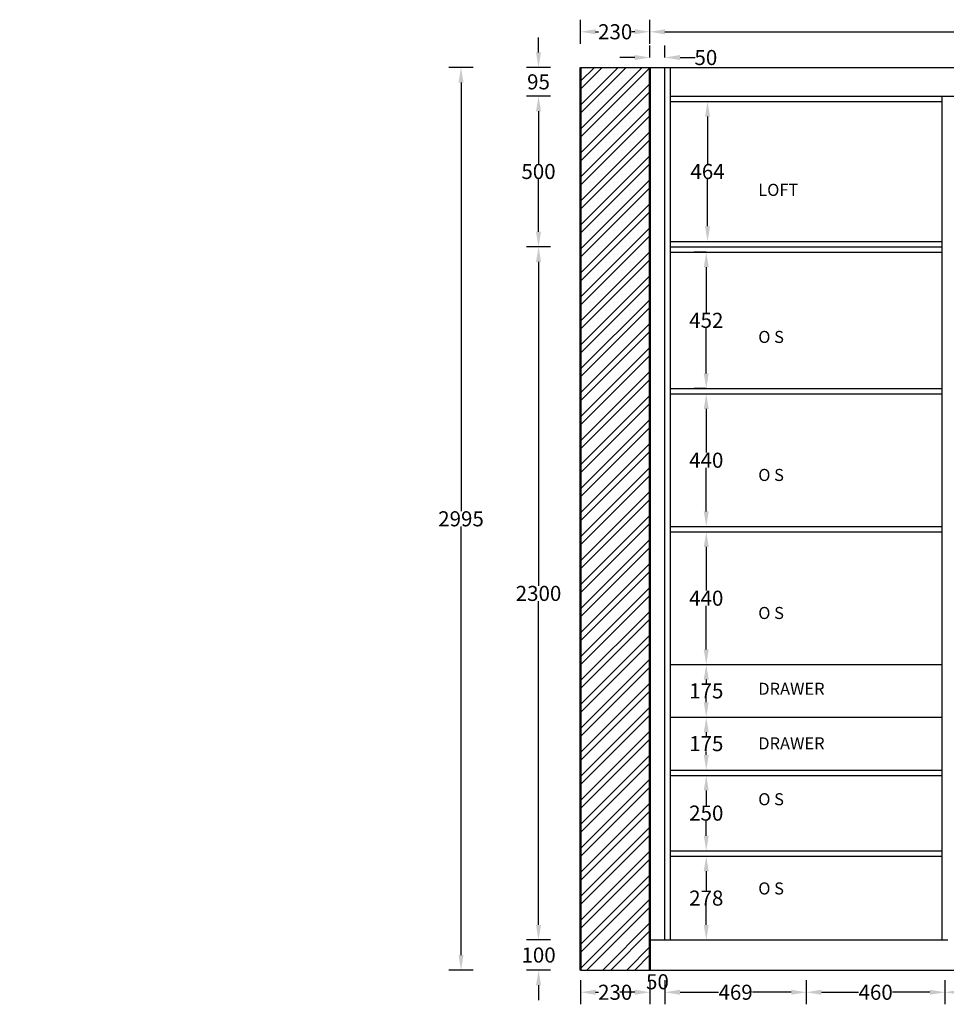
# Model space of a CAD drawing. Units: millimetres. Extents: x -472 to 16192, y -4730 to 4331.
# Tile 4 of 8: x 7860 to 10934, y -4399 to -1132. Entities that reach past the tile are written whole.
import ezdxf

# ---------------------------------------------------------------- set-up
doc = ezdxf.new("R2010")
doc.units = ezdxf.units.MM
doc.header["$MEASUREMENT"] = 0
for name, color, linetype, lineweight in [('A-ANNO-DIMS', 2, 'Continuous', 18), ('A-ANNO-TEXT', 6, 'Continuous', 18), ('A-ELEV', 7, 'Continuous', 25), ('A-WALL', 7, 'Continuous', 50), ('A-WALL-PATT', 8, 'Continuous', 13)]:
    doc.layers.add(name, color=color, linetype=linetype, lineweight=lineweight)
doc.styles.get("Standard").update_dxf_attribs({"font": 'arial.ttf'})
doc.dimstyles.get("Standard").update_dxf_attribs({"dimtxt": 50, "dimasz": 50, "dimexe": 40, "dimexo": 40, "dimgap": 0.09, "dimtad": 0, "dimtih": 1, "dimtoh": 1, "dimdec": 0, "dimzin": 0, "dimdsep": 46, "dimtxsty": 'Standard', "dimcen": 0.09, "dimclrd": 1, "dimclre": 3, "dimclrt": 6, "dimadec": 0, "dimazin": 0, "dimtfac": 1, "dimtdec": 0, "dimtofl": 0, "dimtmove": 0, "dimatfit": 3, "dimfxl": 40, "dimfxlon": 1, "dimtolj": 1, "dimtzin": 0, "dimarcsym": 0})

# ---------------------------------------------------------------- blocks, each defined once
blk = doc.blocks.new('*D44')
at = {"layer": 'A-ANNO-DIMS', "color": 0, "lineweight": -2, "transparency": 16777216}
for p, q in [((9950.7, -1212.4), (9950.7, -1132.4)), ((15090.7, -1212.4), (15090.7, -1132.4)), ((10000.7, -1172.4), (12446, -1172.4)), ((15040.7, -1172.4), (12595.3, -1172.4))]:
    blk.add_line(p, q, dxfattribs=at)
at = {"layer": 'A-ANNO-DIMS', "color": 0, "transparency": 16777216}
for points in [[(10000.7, -1164.1), (10000.7, -1180.8), (9950.7, -1172.4)], [(15040.7, -1164.1), (15040.7, -1180.8), (15090.7, -1172.4)]]:
    blk.add_solid(points, dxfattribs=at)
at = {"layer": 'Defpoints', "color": 0, "transparency": 16777216}
for p in [(15090.7, -1172.4), (9950.7, -1290.9), (15090.7, -1290.9)]:
    blk.add_point(p, dxfattribs=at)
at = {"layer": 'A-ANNO-DIMS', "color": 0, "transparency": 16777216, "insert": (12520.7, -1172.4), "char_height": 50, "attachment_point": 5}
blk.add_mtext('\\A1;5140', dxfattribs=at)
blk = doc.blocks.new('*D46')
at = {"layer": 'A-ANNO-DIMS', "color": 0, "lineweight": -2, "transparency": 16777216}
for p, q in [((9950.7, -1257.8), (9950.7, -1217.8)), ((10000.7, -1257.8), (10000.7, -1217.8)), ((9900.7, -1257.8), (9850.7, -1257.8)), ((10050.7, -1257.8), (10100.7, -1257.8))]:
    blk.add_line(p, q, dxfattribs=at)
at = {"layer": 'A-ANNO-DIMS', "color": 0, "transparency": 16777216}
for points in [[(9900.7, -1249.5), (9900.7, -1266.2), (9950.7, -1257.8)], [(10050.7, -1249.5), (10050.7, -1266.2), (10000.7, -1257.8)]]:
    blk.add_solid(points, dxfattribs=at)
at = {"layer": 'Defpoints', "color": 0, "transparency": 16777216}
for p in [(10000.7, -1257.8), (9950.7, -1290.9), (10000.7, -1290.9)]:
    blk.add_point(p, dxfattribs=at)
at = {"layer": 'A-ANNO-DIMS', "color": 0, "transparency": 16777216, "insert": (10136.5, -1257.8), "char_height": 50, "attachment_point": 5}
blk.add_mtext('\\A1;50', dxfattribs=at)
blk = doc.blocks.new('*D47')
at = {"layer": 'A-ANNO-DIMS', "color": 0, "lineweight": -2, "transparency": 16777216}
for p, q in [((9720.7, -1212.3), (9720.7, -1132.3)), ((9950.7, -1212.3), (9950.7, -1132.3)), ((9770.7, -1172.3), (9780, -1172.3)), ((9900.7, -1172.3), (9891.3, -1172.3))]:
    blk.add_line(p, q, dxfattribs=at)
at = {"layer": 'A-ANNO-DIMS', "color": 0, "transparency": 16777216}
for points in [[(9770.7, -1163.9), (9770.7, -1180.6), (9720.7, -1172.3)], [(9900.7, -1163.9), (9900.7, -1180.6), (9950.7, -1172.3)]]:
    blk.add_solid(points, dxfattribs=at)
at = {"layer": 'Defpoints', "color": 0, "transparency": 16777216}
for p in [(9950.7, -1172.3), (9720.7, -1290.9), (9950.7, -1290.9)]:
    blk.add_point(p, dxfattribs=at)
at = {"layer": 'A-ANNO-DIMS', "color": 0, "transparency": 16777216, "insert": (9835.7, -1172.3), "char_height": 50, "attachment_point": 5}
blk.add_mtext('\\A1;230', dxfattribs=at)
blk = doc.blocks.new('*D48')
at = {"layer": 'A-ANNO-DIMS', "color": 0, "lineweight": -2, "transparency": 16777216}
for p, q in [((9364.2, -1290.9), (9284.2, -1290.9)), ((9324.2, -1340.9), (9324.2, -2762.8)), ((9324.2, -4235.9), (9324.2, -2814)), ((9364.2, -4285.9), (9284.2, -4285.9))]:
    blk.add_line(p, q, dxfattribs=at)
at = {"layer": 'A-ANNO-DIMS', "color": 0, "transparency": 16777216}
for points in [[(9315.8, -1340.9), (9332.5, -1340.9), (9324.2, -1290.9)], [(9315.8, -4235.9), (9332.5, -4235.9), (9324.2, -4285.9)]]:
    blk.add_solid(points, dxfattribs=at)
at = {"layer": 'Defpoints', "color": 0, "transparency": 16777216}
for p in [(9720.7, -1290.9), (9324.2, -4285.9), (9720.7, -4285.9)]:
    blk.add_point(p, dxfattribs=at)
at = {"layer": 'A-ANNO-DIMS', "color": 0, "transparency": 16777216, "insert": (9324.2, -2788.4), "char_height": 50, "attachment_point": 5}
blk.add_mtext('\\A1;2995', dxfattribs=at)
blk = doc.blocks.new('*D49')
at = {"layer": 'A-ANNO-DIMS', "color": 0, "lineweight": -2, "transparency": 16777216}
for p, q in [((9581.5, -4135.9), (9581.5, -4085.9)), ((9621.5, -4185.9), (9541.5, -4185.9)), ((9621.5, -4285.9), (9541.5, -4285.9)), ((9581.5, -4335.9), (9581.5, -4385.9))]:
    blk.add_line(p, q, dxfattribs=at)
at = {"layer": 'A-ANNO-DIMS', "color": 0, "transparency": 16777216}
for points in [[(9573.1, -4135.9), (9589.8, -4135.9), (9581.5, -4185.9)], [(9573.1, -4335.9), (9589.8, -4335.9), (9581.5, -4285.9)]]:
    blk.add_solid(points, dxfattribs=at)
at = {"layer": 'Defpoints', "color": 0, "transparency": 16777216}
for p in [(9950.7, -4185.9), (9581.5, -4285.9), (9950.7, -4285.9)]:
    blk.add_point(p, dxfattribs=at)
at = {"layer": 'A-ANNO-DIMS', "color": 0, "transparency": 16777216, "insert": (9581.5, -4235.9), "char_height": 50, "attachment_point": 5}
blk.add_mtext('\\A1;100', dxfattribs=at)
blk = doc.blocks.new('*D50')
at = {"layer": 'A-ANNO-DIMS', "color": 0, "lineweight": -2, "transparency": 16777216}
for p, q in [((9621.3, -1885.9), (9541.3, -1885.9)), ((9581.3, -1935.9), (9581.3, -3010.3)), ((9581.3, -4135.9), (9581.3, -3061.5)), ((9621.3, -4185.9), (9541.3, -4185.9))]:
    blk.add_line(p, q, dxfattribs=at)
at = {"layer": 'A-ANNO-DIMS', "color": 0, "transparency": 16777216}
for points in [[(9573, -1935.9), (9589.6, -1935.9), (9581.3, -1885.9)], [(9573, -4135.9), (9589.6, -4135.9), (9581.3, -4185.9)]]:
    blk.add_solid(points, dxfattribs=at)
at = {"layer": 'Defpoints', "color": 0, "transparency": 16777216}
for p in [(9950.7, -1885.9), (9581.3, -4185.9), (9950.7, -4185.9)]:
    blk.add_point(p, dxfattribs=at)
at = {"layer": 'A-ANNO-DIMS', "color": 0, "transparency": 16777216, "insert": (9581.3, -3035.9), "char_height": 50, "attachment_point": 5}
blk.add_mtext('\\A1;2300', dxfattribs=at)
blk = doc.blocks.new('*D51')
at = {"layer": 'A-ANNO-DIMS', "color": 0, "lineweight": -2, "transparency": 16777216}
for p, q in [((9621.3, -1385.9), (9541.3, -1385.9)), ((9581.3, -1435.9), (9581.3, -1610.3)), ((9581.3, -1835.9), (9581.3, -1661.5)), ((9621.3, -1885.9), (9541.3, -1885.9))]:
    blk.add_line(p, q, dxfattribs=at)
at = {"layer": 'A-ANNO-DIMS', "color": 0, "transparency": 16777216}
for points in [[(9573, -1435.9), (9589.6, -1435.9), (9581.3, -1385.9)], [(9573, -1835.9), (9589.6, -1835.9), (9581.3, -1885.9)]]:
    blk.add_solid(points, dxfattribs=at)
at = {"layer": 'Defpoints', "color": 0, "transparency": 16777216}
for p in [(10018.7, -1385.9), (9581.3, -1885.9), (9950.7, -1885.9)]:
    blk.add_point(p, dxfattribs=at)
at = {"layer": 'A-ANNO-DIMS', "color": 0, "transparency": 16777216, "insert": (9581.3, -1635.9), "char_height": 50, "attachment_point": 5}
blk.add_mtext('\\A1;500', dxfattribs=at)
blk = doc.blocks.new('*D41')
at = {"layer": 'A-ANNO-DIMS', "color": 0, "lineweight": -2, "transparency": 16777216}
for p, q in [((9581.3, -1240.9), (9581.3, -1190.9)), ((9621.3, -1290.9), (9541.3, -1290.9)), ((9621.3, -1385.9), (9541.3, -1385.9)), ((9581.3, -1435.9), (9581.3, -1485.9))]:
    blk.add_line(p, q, dxfattribs=at)
at = {"layer": 'A-ANNO-DIMS', "color": 0, "transparency": 16777216}
for points in [[(9573, -1240.9), (9589.6, -1240.9), (9581.3, -1290.9)], [(9573, -1435.9), (9589.6, -1435.9), (9581.3, -1385.9)]]:
    blk.add_solid(points, dxfattribs=at)
at = {"layer": 'Defpoints', "color": 0, "transparency": 16777216}
for p in [(9950.7, -1290.9), (9581.3, -1385.9), (9950.7, -1385.9)]:
    blk.add_point(p, dxfattribs=at)
at = {"layer": 'A-ANNO-DIMS', "color": 0, "transparency": 16777216, "insert": (9581.3, -1338.4), "char_height": 50, "attachment_point": 5}
blk.add_mtext('\\A1;95', dxfattribs=at)
blk = doc.blocks.new('*D42')
at = {"layer": 'A-ANNO-DIMS', "color": 0, "lineweight": -2, "transparency": 16777216}
for p, q in [((9720.7, -4319.4), (9720.7, -4399.4)), ((9950.7, -4319.4), (9950.7, -4399.4)), ((9770.7, -4359.4), (9780, -4359.4)), ((9900.7, -4359.4), (9891.3, -4359.4))]:
    blk.add_line(p, q, dxfattribs=at)
at = {"layer": 'A-ANNO-DIMS', "color": 0, "transparency": 16777216}
for points in [[(9770.7, -4351), (9770.7, -4367.7), (9720.7, -4359.4)], [(9900.7, -4351), (9900.7, -4367.7), (9950.7, -4359.4)]]:
    blk.add_solid(points, dxfattribs=at)
at = {"layer": 'Defpoints', "color": 0, "transparency": 16777216}
for p in [(9720.7, -4185.9), (9950.7, -4185.9), (9950.7, -4359.4)]:
    blk.add_point(p, dxfattribs=at)
at = {"layer": 'A-ANNO-DIMS', "color": 0, "transparency": 16777216, "insert": (9835.7, -4359.4), "char_height": 50, "attachment_point": 5}
blk.add_mtext('\\A1;230', dxfattribs=at)
blk = doc.blocks.new('*D43')
at = {"layer": 'A-ANNO-DIMS', "color": 0, "lineweight": -2, "transparency": 16777216}
for p, q in [((9950.7, -4319.4), (9950.7, -4399.4)), ((10000.7, -4319.4), (10000.7, -4399.4)), ((9900.7, -4359.4), (9850.7, -4359.4)), ((10050.7, -4359.4), (10100.7, -4359.4))]:
    blk.add_line(p, q, dxfattribs=at)
at = {"layer": 'A-ANNO-DIMS', "color": 0, "transparency": 16777216}
for points in [[(9900.7, -4351), (9900.7, -4367.7), (9950.7, -4359.4)], [(10050.7, -4351), (10050.7, -4367.7), (10000.7, -4359.4)]]:
    blk.add_solid(points, dxfattribs=at)
at = {"layer": 'Defpoints', "color": 0, "transparency": 16777216}
for p in [(9950.7, -4185.9), (10000.7, -4185.9), (10000.7, -4359.4)]:
    blk.add_point(p, dxfattribs=at)
at = {"layer": 'A-ANNO-DIMS', "color": 0, "transparency": 16777216, "insert": (9975.9, -4324.5), "char_height": 50, "attachment_point": 5}
blk.add_mtext('\\A1;50', dxfattribs=at)
blk = doc.blocks.new('*D52')
at = {"layer": 'A-ANNO-DIMS', "color": 0, "lineweight": -2, "transparency": 16777216}
for p, q in [((10000.7, -4319.4), (10000.7, -4399.4)), ((10469.7, -4319.4), (10469.7, -4399.4)), ((10050.7, -4359.4), (10178.8, -4359.4)), ((10419.7, -4359.4), (10291.5, -4359.4))]:
    blk.add_line(p, q, dxfattribs=at)
at = {"layer": 'A-ANNO-DIMS', "color": 0, "transparency": 16777216}
for points in [[(10050.7, -4351), (10050.7, -4367.7), (10000.7, -4359.4)], [(10419.7, -4351), (10419.7, -4367.7), (10469.7, -4359.4)]]:
    blk.add_solid(points, dxfattribs=at)
at = {"layer": 'Defpoints', "color": 0, "transparency": 16777216}
for p in [(10000.7, -4185.9), (10469.7, -4185.9), (10469.7, -4359.4)]:
    blk.add_point(p, dxfattribs=at)
at = {"layer": 'A-ANNO-DIMS', "color": 0, "transparency": 16777216, "insert": (10235.2, -4359.4), "char_height": 50, "attachment_point": 5}
blk.add_mtext('\\A1;469', dxfattribs=at)
blk = doc.blocks.new('*D53')
at = {"layer": 'A-ANNO-DIMS', "color": 0, "lineweight": -2, "transparency": 16777216}
for p, q in [((10469.7, -4319.4), (10469.7, -4399.4)), ((10929.7, -4319.4), (10929.7, -4399.4)), ((10519.7, -4359.4), (10643.4, -4359.4)), ((10879.7, -4359.4), (10755.9, -4359.4))]:
    blk.add_line(p, q, dxfattribs=at)
at = {"layer": 'A-ANNO-DIMS', "color": 0, "transparency": 16777216}
for points in [[(10519.7, -4351), (10519.7, -4367.7), (10469.7, -4359.4)], [(10879.7, -4351), (10879.7, -4367.7), (10929.7, -4359.4)]]:
    blk.add_solid(points, dxfattribs=at)
at = {"layer": 'Defpoints', "color": 0, "transparency": 16777216}
for p in [(10469.7, -4185.9), (10929.7, -4185.9), (10929.7, -4359.4)]:
    blk.add_point(p, dxfattribs=at)
at = {"layer": 'A-ANNO-DIMS', "color": 0, "transparency": 16777216, "insert": (10699.7, -4359.4), "char_height": 50, "attachment_point": 5}
blk.add_mtext('\\A1;460', dxfattribs=at)
blk = doc.blocks.new('*D54')
at = {"layer": 'A-ANNO-DIMS', "color": 0, "lineweight": -2, "transparency": 16777216}
for p, q in [((10929.7, -4319.4), (10929.7, -4399.4)), ((11389.7, -4319.4), (11389.7, -4399.4)), ((10979.7, -4359.4), (11103.4, -4359.4)), ((11339.7, -4359.4), (11215.9, -4359.4))]:
    blk.add_line(p, q, dxfattribs=at)
at = {"layer": 'A-ANNO-DIMS', "color": 0, "transparency": 16777216}
for points in [[(10979.7, -4351), (10979.7, -4367.7), (10929.7, -4359.4)], [(11339.7, -4351), (11339.7, -4367.7), (11389.7, -4359.4)]]:
    blk.add_solid(points, dxfattribs=at)
at = {"layer": 'Defpoints', "color": 0, "transparency": 16777216}
for p in [(10929.7, -4185.9), (11389.7, -4185.9), (11389.7, -4359.4)]:
    blk.add_point(p, dxfattribs=at)
at = {"layer": 'A-ANNO-DIMS', "color": 0, "transparency": 16777216, "insert": (11159.7, -4359.4), "char_height": 50, "attachment_point": 5}
blk.add_mtext('\\A1;460', dxfattribs=at)
blk = doc.blocks.new('*D65')
at = {"layer": 'A-ANNO-DIMS', "color": 0, "lineweight": -2, "transparency": 16777216}
for p, q in [((10097.8, -3907.9), (10177.8, -3907.9)), ((10137.8, -3957.9), (10137.8, -4021.3)), ((10137.8, -4135.9), (10137.8, -4072.5)), ((10097.8, -4185.9), (10177.8, -4185.9))]:
    blk.add_line(p, q, dxfattribs=at)
at = {"layer": 'A-ANNO-DIMS', "color": 0, "transparency": 16777216}
for points in [[(10129.5, -3957.9), (10146.1, -3957.9), (10137.8, -3907.9)], [(10129.5, -4135.9), (10146.1, -4135.9), (10137.8, -4185.9)]]:
    blk.add_solid(points, dxfattribs=at)
at = {"layer": 'Defpoints', "color": 0, "transparency": 16777216}
for p in [(10018.7, -3907.9), (10137.8, -3907.9), (10018.7, -4185.9)]:
    blk.add_point(p, dxfattribs=at)
at = {"layer": 'A-ANNO-DIMS', "color": 0, "transparency": 16777216, "insert": (10137.8, -4046.9), "char_height": 50, "attachment_point": 5}
blk.add_mtext('\\A1;278', dxfattribs=at)
blk = doc.blocks.new('*D66')
at = {"layer": 'A-ANNO-DIMS', "color": 0, "lineweight": -2, "transparency": 16777216}
for p, q in [((10137.8, -3639.9), (10177.8, -3639.9)), ((10137.8, -3689.9), (10137.8, -3739.3)), ((10137.8, -3839.9), (10137.8, -3790.5)), ((10137.8, -3889.9), (10177.8, -3889.9))]:
    blk.add_line(p, q, dxfattribs=at)
at = {"layer": 'A-ANNO-DIMS', "color": 0, "transparency": 16777216}
for points in [[(10129.5, -3689.9), (10146.1, -3689.9), (10137.8, -3639.9)], [(10129.5, -3839.9), (10146.1, -3839.9), (10137.8, -3889.9)]]:
    blk.add_solid(points, dxfattribs=at)
at = {"layer": 'Defpoints', "color": 0, "transparency": 16777216}
for p in [(10137.8, -3639.9), (10137.8, -3639.9), (10137.8, -3889.9)]:
    blk.add_point(p, dxfattribs=at)
at = {"layer": 'A-ANNO-DIMS', "color": 0, "transparency": 16777216, "insert": (10137.8, -3764.9), "char_height": 50, "attachment_point": 5}
blk.add_mtext('\\A1;250', dxfattribs=at)
blk = doc.blocks.new('*D67')
at = {"layer": 'A-ANNO-DIMS', "color": 0, "lineweight": -2, "transparency": 16777216}
for p, q in [((10137.8, -3446.9), (10177.8, -3446.9)), ((10137.8, -3496.9), (10137.8, -3508.8)), ((10137.8, -3571.9), (10137.8, -3560)), ((10137.8, -3621.9), (10177.8, -3621.9))]:
    blk.add_line(p, q, dxfattribs=at)
at = {"layer": 'A-ANNO-DIMS', "color": 0, "transparency": 16777216}
for points in [[(10129.5, -3496.9), (10146.1, -3496.9), (10137.8, -3446.9)], [(10129.5, -3571.9), (10146.1, -3571.9), (10137.8, -3621.9)]]:
    blk.add_solid(points, dxfattribs=at)
at = {"layer": 'Defpoints', "color": 0, "transparency": 16777216}
for p in [(10137.8, -3446.9), (10137.8, -3446.9), (10137.8, -3621.9)]:
    blk.add_point(p, dxfattribs=at)
at = {"layer": 'A-ANNO-DIMS', "color": 0, "transparency": 16777216, "insert": (10137.8, -3534.4), "char_height": 50, "attachment_point": 5}
blk.add_mtext('\\A1;175', dxfattribs=at)
blk = doc.blocks.new('*D68')
at = {"layer": 'A-ANNO-DIMS', "color": 0, "lineweight": -2, "transparency": 16777216}
for p, q in [((10137.8, -3271.9), (10177.8, -3271.9)), ((10137.8, -3321.9), (10137.8, -3333.8)), ((10137.8, -3396.9), (10137.8, -3385)), ((10137.8, -3446.9), (10177.8, -3446.9))]:
    blk.add_line(p, q, dxfattribs=at)
at = {"layer": 'A-ANNO-DIMS', "color": 0, "transparency": 16777216}
for points in [[(10129.5, -3321.9), (10146.1, -3321.9), (10137.8, -3271.9)], [(10129.5, -3396.9), (10146.1, -3396.9), (10137.8, -3446.9)]]:
    blk.add_solid(points, dxfattribs=at)
at = {"layer": 'Defpoints', "color": 0, "transparency": 16777216}
for p in [(10137.8, -3271.9), (10137.8, -3271.9), (10137.8, -3446.9)]:
    blk.add_point(p, dxfattribs=at)
at = {"layer": 'A-ANNO-DIMS', "color": 0, "transparency": 16777216, "insert": (10137.8, -3359.4), "char_height": 50, "attachment_point": 5}
blk.add_mtext('\\A1;175', dxfattribs=at)
blk = doc.blocks.new('*D69')
at = {"layer": 'A-ANNO-DIMS', "color": 0, "lineweight": -2, "transparency": 16777216}
for p, q in [((10137.8, -2831.9), (10177.8, -2831.9)), ((10137.8, -2881.9), (10137.8, -3026.3)), ((10137.8, -3221.9), (10137.8, -3077.5)), ((10137.8, -3271.9), (10177.8, -3271.9))]:
    blk.add_line(p, q, dxfattribs=at)
at = {"layer": 'A-ANNO-DIMS', "color": 0, "transparency": 16777216}
for points in [[(10129.5, -2881.9), (10146.1, -2881.9), (10137.8, -2831.9)], [(10129.5, -3221.9), (10146.1, -3221.9), (10137.8, -3271.9)]]:
    blk.add_solid(points, dxfattribs=at)
at = {"layer": 'Defpoints', "color": 0, "transparency": 16777216}
for p in [(10137.8, -2831.9), (10137.8, -2831.9), (10137.8, -3271.9)]:
    blk.add_point(p, dxfattribs=at)
at = {"layer": 'A-ANNO-DIMS', "color": 0, "transparency": 16777216, "insert": (10137.8, -3051.9), "char_height": 50, "attachment_point": 5}
blk.add_mtext('\\A1;440', dxfattribs=at)
blk = doc.blocks.new('*D70')
at = {"layer": 'A-ANNO-DIMS', "color": 0, "lineweight": -2, "transparency": 16777216}
for p, q in [((10137.8, -2373.9), (10177.8, -2373.9)), ((10137.8, -2423.9), (10137.8, -2568.3)), ((10137.8, -2763.9), (10137.8, -2619.5)), ((10137.8, -2813.9), (10177.8, -2813.9))]:
    blk.add_line(p, q, dxfattribs=at)
at = {"layer": 'A-ANNO-DIMS', "color": 0, "transparency": 16777216}
for points in [[(10129.5, -2423.9), (10146.1, -2423.9), (10137.8, -2373.9)], [(10129.5, -2763.9), (10146.1, -2763.9), (10137.8, -2813.9)]]:
    blk.add_solid(points, dxfattribs=at)
at = {"layer": 'Defpoints', "color": 0, "transparency": 16777216}
for p in [(10137.8, -2373.9), (10137.8, -2373.9), (10137.8, -2813.9)]:
    blk.add_point(p, dxfattribs=at)
at = {"layer": 'A-ANNO-DIMS', "color": 0, "transparency": 16777216, "insert": (10137.8, -2593.9), "char_height": 50, "attachment_point": 5}
blk.add_mtext('\\A1;440', dxfattribs=at)
blk = doc.blocks.new('*D71')
at = {"layer": 'A-ANNO-DIMS', "color": 0, "lineweight": -2, "transparency": 16777216}
for p, q in [((10137.8, -1903.9), (10097.8, -1903.9)), ((10137.8, -1953.9), (10137.8, -2104.3)), ((10137.8, -2305.9), (10137.8, -2155.5)), ((10137.8, -2355.9), (10097.8, -2355.9))]:
    blk.add_line(p, q, dxfattribs=at)
at = {"layer": 'A-ANNO-DIMS', "color": 0, "transparency": 16777216}
for points in [[(10129.5, -1953.9), (10146.1, -1953.9), (10137.8, -1903.9)], [(10129.5, -2305.9), (10146.1, -2305.9), (10137.8, -2355.9)]]:
    blk.add_solid(points, dxfattribs=at)
at = {"layer": 'Defpoints', "color": 0, "transparency": 16777216}
for p in [(10137.8, -1903.9), (10143, -1903.9), (10143, -2355.9)]:
    blk.add_point(p, dxfattribs=at)
at = {"layer": 'A-ANNO-DIMS', "color": 0, "transparency": 16777216, "insert": (10137.8, -2129.9), "char_height": 50, "attachment_point": 5}
blk.add_mtext('\\A1;452', dxfattribs=at)
blk = doc.blocks.new('*D72')
at = {"layer": 'A-ANNO-DIMS', "color": 0, "lineweight": -2, "transparency": 16777216}
for p, q in [((10142, -1403.9), (10182, -1403.9)), ((10142, -1453.9), (10142, -1610.3)), ((10142, -1817.9), (10142, -1661.5)), ((10142, -1867.9), (10182, -1867.9))]:
    blk.add_line(p, q, dxfattribs=at)
at = {"layer": 'A-ANNO-DIMS', "color": 0, "transparency": 16777216}
for points in [[(10133.6, -1453.9), (10150.3, -1453.9), (10142, -1403.9)], [(10133.6, -1817.9), (10150.3, -1817.9), (10142, -1867.9)]]:
    blk.add_solid(points, dxfattribs=at)
at = {"layer": 'Defpoints', "color": 0, "transparency": 16777216}
for p in [(10137.8, -1403.9), (10142, -1403.9), (10137.8, -1867.9)]:
    blk.add_point(p, dxfattribs=at)
at = {"layer": 'A-ANNO-DIMS', "color": 0, "transparency": 16777216, "insert": (10142, -1635.9), "char_height": 50, "attachment_point": 5}
blk.add_mtext('\\A1;464', dxfattribs=at)
blk = doc.blocks.new('*D100')
at = {"layer": 'A-ANNO-DIMS', "color": 1, "lineweight": -2, "transparency": 16777216}
for p, q in [((16116.7, -1835.9), (16116.7, -1785.9)), ((16116.7, -2035.9), (16116.7, -2085.9))]:
    blk.add_line(p, q, dxfattribs=at)
at = {"layer": 'A-ANNO-DIMS', "color": 3, "lineweight": -2, "transparency": 16777216}
for p, q in [((16076.7, -1885.9), (16156.7, -1885.9)), ((16076.7, -1985.9), (16156.7, -1985.9))]:
    blk.add_line(p, q, dxfattribs=at)
at = {"layer": 'A-ANNO-DIMS', "color": 1, "transparency": 16777216}
for points in [[(16108.3, -1835.9), (16125, -1835.9), (16116.7, -1885.9)], [(16108.3, -2035.9), (16125, -2035.9), (16116.7, -1985.9)]]:
    blk.add_solid(points, dxfattribs=at)
at = {"layer": 'Defpoints', "color": 0, "transparency": 16777216}
for p in [(5309, -1885.9), (5209, -1985.9), (16116.7, -1985.9)]:
    blk.add_point(p, dxfattribs=at)
at = {"layer": 'A-ANNO-DIMS', "color": 6, "transparency": 16777216, "insert": (16116.7, -1935.9), "char_height": 50, "attachment_point": 5}
blk.add_mtext('\\A1;100', dxfattribs=at)
blk = doc.blocks.new('*D101')
at = {"layer": 'A-ANNO-DIMS', "color": 3, "lineweight": -2, "transparency": 16777216}
for p, q in [((16076.7, -1985.9), (16156.7, -1985.9)), ((16076.7, -3535.9), (16156.7, -3535.9))]:
    blk.add_line(p, q, dxfattribs=at)
at = {"layer": 'A-ANNO-DIMS', "color": 1, "lineweight": -2, "transparency": 16777216}
for p, q in [((16116.7, -2035.9), (16116.7, -2735.3)), ((16116.7, -3485.9), (16116.7, -2786.5))]:
    blk.add_line(p, q, dxfattribs=at)
at = {"layer": 'A-ANNO-DIMS', "color": 1, "transparency": 16777216}
for points in [[(16108.3, -2035.9), (16125, -2035.9), (16116.7, -1985.9)], [(16108.3, -3485.9), (16125, -3485.9), (16116.7, -3535.9)]]:
    blk.add_solid(points, dxfattribs=at)
at = {"layer": 'Defpoints', "color": 0, "transparency": 16777216}
for p in [(5209, -1985.9), (5209, -3535.9), (16116.7, -3535.9)]:
    blk.add_point(p, dxfattribs=at)
at = {"layer": 'A-ANNO-DIMS', "color": 6, "transparency": 16777216, "insert": (16116.7, -2760.9), "char_height": 50, "attachment_point": 5}
blk.add_mtext('\\A1;1550', dxfattribs=at)
blk = doc.blocks.new('*D102')
at = {"layer": 'A-ANNO-DIMS', "color": 3, "lineweight": -2, "transparency": 16777216}
for p, q in [((16076.7, -2035.9), (16156.7, -2035.9)), ((16076.7, -3485.9), (16156.7, -3485.9))]:
    blk.add_line(p, q, dxfattribs=at)
at = {"layer": 'A-ANNO-DIMS', "color": 1, "lineweight": -2, "transparency": 16777216}
for p, q in [((16116.7, -2085.9), (16116.7, -2735.3)), ((16116.7, -3435.9), (16116.7, -2786.5))]:
    blk.add_line(p, q, dxfattribs=at)
at = {"layer": 'A-ANNO-DIMS', "color": 1, "transparency": 16777216}
for points in [[(16108.3, -2085.9), (16125, -2085.9), (16116.7, -2035.9)], [(16108.3, -3435.9), (16125, -3435.9), (16116.7, -3485.9)]]:
    blk.add_solid(points, dxfattribs=at)
at = {"layer": 'Defpoints', "color": 0, "transparency": 16777216}
for p in [(5159, -2035.9), (5159, -3485.9), (16116.7, -3485.9)]:
    blk.add_point(p, dxfattribs=at)
at = {"layer": 'A-ANNO-DIMS', "color": 6, "transparency": 16777216, "insert": (16116.7, -2760.9), "char_height": 50, "attachment_point": 5}
blk.add_mtext('\\A1;1450', dxfattribs=at)
blk = doc.blocks.new('*D103')
at = {"layer": 'A-ANNO-DIMS', "color": 1, "lineweight": -2, "transparency": 16777216}
for p, q in [((16116.7, -3485.9), (16116.7, -3435.9)), ((16116.7, -3685.9), (16116.7, -3735.9))]:
    blk.add_line(p, q, dxfattribs=at)
at = {"layer": 'A-ANNO-DIMS', "color": 3, "lineweight": -2, "transparency": 16777216}
for p, q in [((16076.7, -3535.9), (16156.7, -3535.9)), ((16076.7, -3635.9), (16156.7, -3635.9))]:
    blk.add_line(p, q, dxfattribs=at)
at = {"layer": 'A-ANNO-DIMS', "color": 1, "transparency": 16777216}
for points in [[(16108.3, -3485.9), (16125, -3485.9), (16116.7, -3535.9)], [(16108.3, -3685.9), (16125, -3685.9), (16116.7, -3635.9)]]:
    blk.add_solid(points, dxfattribs=at)
at = {"layer": 'Defpoints', "color": 0, "transparency": 16777216}
for p in [(5209, -3535.9), (5309, -3635.9), (16116.7, -3635.9)]:
    blk.add_point(p, dxfattribs=at)
at = {"layer": 'A-ANNO-DIMS', "color": 6, "transparency": 16777216, "insert": (16116.7, -3585.9), "char_height": 50, "attachment_point": 5}
blk.add_mtext('\\A1;100', dxfattribs=at)
blk = doc.blocks.new('*D104')
at = {"layer": 'A-ANNO-DIMS', "color": 1, "lineweight": -2, "transparency": 16777216}
for p, q in [((16116.7, -3585.9), (16116.7, -3535.9)), ((16116.7, -3735.9), (16116.7, -3785.9)), ((16116.7, -3785.9), (16066.7, -3785.9))]:
    blk.add_line(p, q, dxfattribs=at)
at = {"layer": 'A-ANNO-DIMS', "color": 3, "lineweight": -2, "transparency": 16777216}
for p, q in [((16076.7, -3635.9), (16156.7, -3635.9)), ((16076.7, -3685.9), (16156.7, -3685.9))]:
    blk.add_line(p, q, dxfattribs=at)
at = {"layer": 'A-ANNO-DIMS', "color": 1, "transparency": 16777216}
for points in [[(16108.3, -3585.9), (16125, -3585.9), (16116.7, -3635.9)], [(16108.3, -3735.9), (16125, -3735.9), (16116.7, -3685.9)]]:
    blk.add_solid(points, dxfattribs=at)
at = {"layer": 'Defpoints', "color": 0, "transparency": 16777216}
for p in [(5309, -3635.9), (5309, -3685.9), (16116.7, -3685.9)]:
    blk.add_point(p, dxfattribs=at)
at = {"layer": 'A-ANNO-DIMS', "color": 6, "transparency": 16777216, "insert": (16030.8, -3785.9), "char_height": 50, "attachment_point": 5}
blk.add_mtext('\\A1;50', dxfattribs=at)

msp = doc.modelspace()

# ---------------------------------------------------------------- hatches: boundary and pattern name
at = {"layer": 'A-WALL-PATT'}
h = msp.add_hatch(dxfattribs=at)
h.set_pattern_fill('ANSI32', color=256, scale=150)
h.paths.add_polyline_path([(9720.7, -1290.9), (9720.7, -4285.9), (9950.7, -4285.9), (9950.7, -4185.9), (9950.7, -1885.9), (9950.7, -1290.9)])
h.paths.add_polyline_path([(5370, -4285.9), (5600, -4285.9), (5600, -1290.9), (5370, -1290.9)])
h.paths.add_polyline_path([(15320.7, -1290.9), (15090.7, -1290.9), (15090.7, -4285.9), (15320.7, -4285.9)])
h.paths.add_polyline_path([(0, -4285.9), (230, -4285.9), (230, -4185.9), (230, -1885.9), (230, -1290.9), (0, -1290.9)])

# ---------------------------------------------------------------- linework, layer by layer
at = {"layer": 'A-ELEV'}
for p, q in [((9720.7, -1290.9), (15320.7, -1290.9)), ((10000.7, -4185.9), (10000.7, -1290.9)), ((10018.7, -4185.9), (10018.7, -1290.9)), ((10018.7, -1385.9), (12769.7, -1385.9)), ((10018.7, -1885.9), (10018.7, -1385.9)), ((10018.7, -1403.9), (10920.7, -1403.9)), ((10920.7, -1885.9), (10920.7, -1385.9)), ((10018.7, -1867.9), (10920.7, -1867.9)), ((10018.7, -1885.9), (10920.7, -1885.9)), ((10920.7, -4185.9), (10920.7, -1885.9)), ((10018.7, -1903.9), (10920.7, -1903.9)), ((10018.7, -2355.9), (10920.7, -2355.9)), ((10018.7, -2373.9), (10920.7, -2373.9)), ((10018.7, -2813.9), (10920.7, -2813.9)), ((10018.7, -2831.9), (10920.7, -2831.9)), ((10018.7, -3271.9), (10920.7, -3271.9)), ((10018.7, -3446.9), (10920.7, -3446.9)), ((10018.7, -3621.9), (10920.7, -3621.9)), ((10018.7, -3639.9), (10920.7, -3639.9)), ((10018.7, -3889.9), (10920.7, -3889.9)), ((10018.7, -3907.9), (10920.7, -3907.9)), ((9950.7, -4185.9), (10938.7, -4185.9)), ((9720.7, -4285.9), (15320.7, -4285.9))]:
    msp.add_line(p, q, dxfattribs=at)
at = {"layer": 'A-WALL'}
for p, q in [((9720.7, -4285.9), (9720.7, -1290.9)), ((9950.7, -1885.9), (9950.7, -1290.9)), ((9950.7, -4185.9), (9950.7, -1885.9)), ((9950.7, -4285.9), (9950.7, -4185.9))]:
    msp.add_line(p, q, dxfattribs=at)

# ---------------------------------------------------------------- texts
at = {"layer": 'A-ANNO-TEXT', "char_height": 40, "attachment_point": 1}
for s, insert in [('LOFT', (10310.3, -1676.9)), ('O S', (10310.3, -2164.9)), ('O S', (10310.3, -2622.9)), ('O S', (10310.3, -3080.9)), ('DRAWER', (10310.3, -3332.4)), ('DRAWER', (10310.3, -3513.5)), ('O S', (10310.3, -3698.9)), ('O S', (10310.3, -3994.9))]:
    msp.add_mtext_dynamic_manual_height_columns(s, width=327.678, gutter_width=1, heights=[0], dxfattribs=dict(at, insert=insert))

# ---------------------------------------------------------------- dimensions: what is measured, and where the dimension line sits
at = {"layer": 'A-ANNO-DIMS'}
for base, p1, p2, override, picture, middle in [((9950.7, -1172.3), (9720.7, -1290.9), (9950.7, -1290.9), {"dimclrd": 0, "dimclre": 0, "dimclrt": 0}, '*D47', (9835.7, -1172.3)), ((15090.7, -1172.4), (9950.7, -1290.9), (15090.7, -1290.9), {"dimclrd": 0, "dimclre": 0, "dimclrt": 0}, '*D44', (12520.7, -1172.4)), ((10000.7, -1257.8), (9950.7, -1290.9), (10000.7, -1290.9), {"dimclrd": 0, "dimclre": 0, "dimclrt": 0}, '*D46', (10136.5, -1257.8)), ((9950.7, -4359.4), (9720.7, -4185.9), (9950.7, -4185.9), {"dimclrd": 0, "dimclre": 0, "dimclrt": 0}, '*D42', (9835.7, -4359.4)), ((10469.7, -4359.4), (10000.7, -4185.9), (10469.7, -4185.9), {"dimclrd": 0, "dimclre": 0, "dimclrt": 0, "dimtmove": 1}, '*D52', (10235.2, -4359.4)), ((10929.7, -4359.4), (10469.7, -4185.9), (10929.7, -4185.9), {"dimclrd": 0, "dimclre": 0, "dimclrt": 0, "dimtmove": 1}, '*D53', (10699.7, -4359.4)), ((11389.7, -4359.4), (10929.7, -4185.9), (11389.7, -4185.9), {"dimclrd": 0, "dimclre": 0, "dimclrt": 0, "dimtmove": 1}, '*D54', (11159.7, -4359.4))]:
    dim = msp.add_linear_dim(base=base, p1=p1, p2=p2, dimstyle='Standard', override=override, dxfattribs=at)
    dim.commit()
    dim.dimension.update_dxf_attribs({"geometry": picture, "text_midpoint": middle})
for base, p1, p2, override, picture, middle in [((9581.3, -1385.9), (9950.7, -1290.9), (9950.7, -1385.9), {"dimclrd": 0, "dimclre": 0, "dimclrt": 0}, '*D41', (9581.3, -1338.4)), ((9324.2, -4285.9), (9720.7, -1290.9), (9720.7, -4285.9), {"dimclrd": 0, "dimclre": 0, "dimclrt": 0}, '*D48', (9324.2, -2788.4)), ((9581.3, -1885.9), (10018.7, -1385.9), (9950.7, -1885.9), {"dimclrd": 0, "dimclre": 0, "dimclrt": 0}, '*D51', (9581.3, -1635.9)), ((10142, -1403.9), (10137.8, -1867.9), (10137.8, -1403.9), {"dimclrd": 0, "dimclre": 0, "dimclrt": 0}, '*D72', (10142, -1635.9)), ((16116.7, -1985.9), (5309, -1885.9), (5209, -1985.9), {"dimdec": 0, "dimlfac": 1, "dimrnd": 0, "dimzin": 0, "dimdsep": 46, "dimlunit": 2}, '*D100', (16116.7, -1935.9)), ((9581.3, -4185.9), (9950.7, -1885.9), (9950.7, -4185.9), {"dimclrd": 0, "dimclre": 0, "dimclrt": 0}, '*D50', (9581.3, -3035.9)), ((10137.8, -1903.9), (10143, -2355.9), (10143, -1903.9), {"dimclrd": 0, "dimclre": 0, "dimclrt": 0}, '*D71', (10137.8, -2129.9)), ((16116.7, -3535.9), (5209, -1985.9), (5209, -3535.9), {"dimdec": 0, "dimlfac": 1, "dimrnd": 0, "dimzin": 0, "dimdsep": 46, "dimlunit": 2}, '*D101', (16116.7, -2760.9)), ((16116.7, -3485.9), (5159, -2035.9), (5159, -3485.9), {"dimdec": 0, "dimlfac": 1, "dimrnd": 0, "dimzin": 0, "dimdsep": 46, "dimlunit": 2}, '*D102', (16116.7, -2760.9)), ((10137.8, -2373.9), (10137.8, -2813.9), (10137.8, -2373.9), {"dimclrd": 0, "dimclre": 0, "dimclrt": 0}, '*D70', (10137.8, -2593.9)), ((10137.8, -2831.9), (10137.8, -3271.9), (10137.8, -2831.9), {"dimclrd": 0, "dimclre": 0, "dimclrt": 0}, '*D69', (10137.8, -3051.9)), ((10137.8, -3271.9), (10137.8, -3446.9), (10137.8, -3271.9), {"dimclrd": 0, "dimclre": 0, "dimclrt": 0}, '*D68', (10137.8, -3359.4)), ((16116.7, -3635.9), (5209, -3535.9), (5309, -3635.9), {"dimdec": 0, "dimlfac": 1, "dimrnd": 0, "dimzin": 0, "dimdsep": 46, "dimlunit": 2}, '*D103', (16116.7, -3585.9)), ((10137.8, -3446.9), (10137.8, -3621.9), (10137.8, -3446.9), {"dimclrd": 0, "dimclre": 0, "dimclrt": 0}, '*D67', (10137.8, -3534.4)), ((16116.7, -3685.9), (5309, -3635.9), (5309, -3685.9), {"dimdec": 0, "dimlfac": 1, "dimrnd": 0, "dimzin": 0, "dimdsep": 46, "dimlunit": 2}, '*D104', (16030.8, -3785.9)), ((10137.8, -3639.9), (10137.8, -3889.9), (10137.8, -3639.9), {"dimclrd": 0, "dimclre": 0, "dimclrt": 0}, '*D66', (10137.8, -3764.9)), ((10137.8, -3907.9), (10018.7, -4185.9), (10018.7, -3907.9), {"dimclrd": 0, "dimclre": 0, "dimclrt": 0}, '*D65', (10137.8, -4046.9)), ((9581.5, -4285.9), (9950.7, -4185.9), (9950.7, -4285.9), {"dimclrd": 0, "dimclre": 0, "dimclrt": 0}, '*D49', (9581.5, -4235.9))]:
    dim = msp.add_linear_dim(base=base, p1=p1, p2=p2, angle=90, dimstyle='Standard', override=override, dxfattribs=at)
    dim.commit()
    dim.dimension.update_dxf_attribs({"geometry": picture, "text_midpoint": middle})
dim = msp.add_linear_dim(base=(10000.7, -4359.4), p1=(9950.7, -4185.9), p2=(10000.7, -4185.9), dimstyle='Standard', override={"dimclrd": 0, "dimclre": 0, "dimclrt": 0, "dimtmove": 2}, dxfattribs=at)
dim.commit()
dim.dimension.update_dxf_attribs({"geometry": '*D43', "text_midpoint": (9975.9, -4324.5), "dimtype": 160})

doc.saveas('drawing.dxf')
